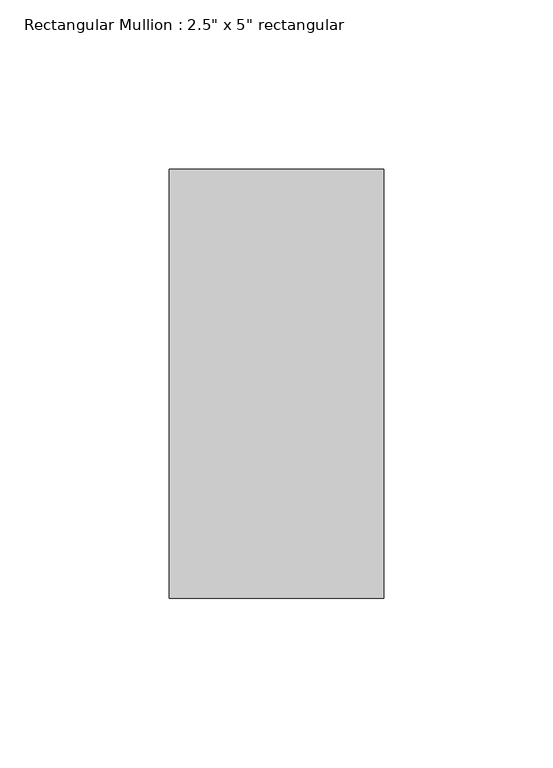
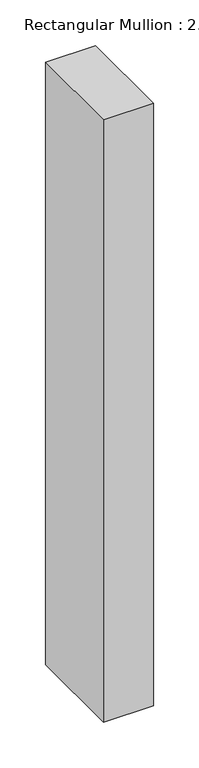
"""IFC4 building model written with IfcOpenShell, lengths in millimetres: member geometry."""

from ifc_helpers import new_model, si_unit, frame, origin, place, context, project, spatial, polyline, outline, extrude, source, transform, mapped, element, save


def member_cb8890cf(model_context):
    return source(origin(), model_context, "Body", "SweptSolid", [
        extrude(outline(polyline([(0.0, 63.5), (0.0, -63.5), (-63.5, -63.5), (-63.5, 63.5), (0.0, 63.5)])), frame((0.0, 0.0, -806.1882113), z_axis=(0.0, 0.0, 1.0), x_axis=(1.0, 0.0, 0.0)), (0.0, 0.0, 1.0), 806.1882113),
    ])


if __name__ == "__main__":
    model = new_model("IFC4")
    model_context = context("Model", 3, world=origin())
    ifc_project = project(units=[si_unit("LENGTHUNIT", "METRE", prefix="MILLI")], contexts=[model_context])
    site = spatial("IfcSite", under=ifc_project)
    building = spatial("IfcBuilding", under=site)
    placement = place(None, origin())
    member_shape = member_cb8890cf(model_context)
    element("IfcMember", 1, ObjectType="Rectangular Mullion : 2.5\" x 5\" rectangular", at=placement, inside=building, context=model_context, shape_type="MappedRepresentation", body=[
        mapped(member_shape, transform((0.0, 0.0, 0.0), x_axis=(1.0, 0.0, 0.0), y_axis=(0.0, 1.0, 0.0), z_axis=(0.0, 0.0, 1.0))),
    ])
    save(model, "model.ifc")

# Revit data of these elements
# Type "Rectangular Mullion : 2.5\" x 5\" rectangular"
#   built-in parameter 1007304 = 0.416667 (stored number, unit not read)
#   built-in parameter 1007301 = 0.104167 (stored number, unit not read)
#   built-in parameter 1007300 = 0.104167 (stored number, unit not read)
# Element 1 (IfcMember, "Rectangular Mullion : 2.5\" x 5\" rectangular")
#   Materials on its faces: "Aluminum"
# Materials
#   "Aluminum": class "Metal", colour RGB 247 247 247, transparency 0, Description = "Aluminum 6061", Cost = 0
